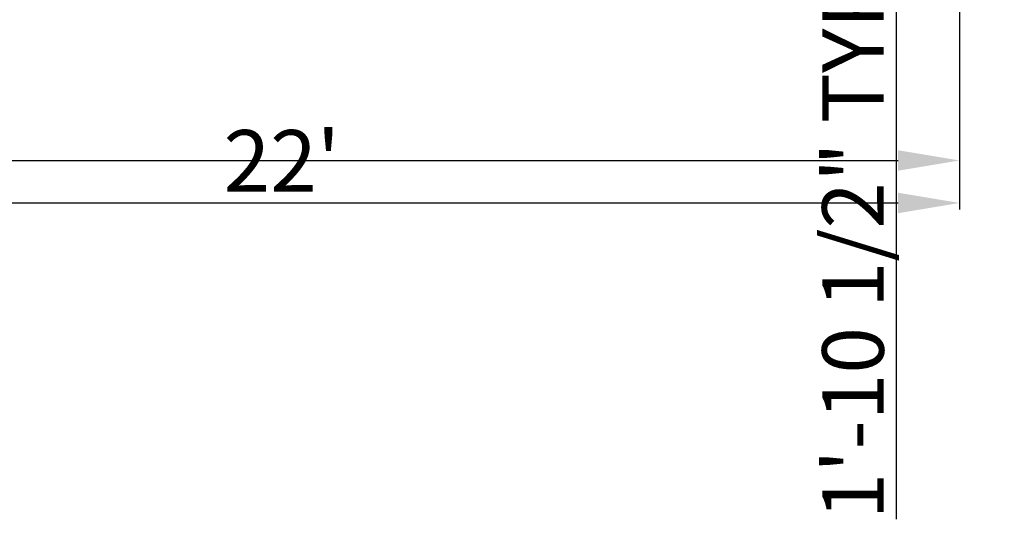
# Model space of a CAD drawing. Units: inches. Extents: x 2083 to 3317, y 1141 to 2115.
# Tile 117 of 256: x 2944 to 3136, y 1141 to 1238. Entities that reach past the tile are written whole.
import ezdxf

# ---------------------------------------------------------------- set-up
doc = ezdxf.new("R2010")
doc.units = ezdxf.units.IN
doc.layers.add('A-ANNO-DIMS', color=2, linetype='Continuous', lineweight=18)
doc.styles.get("Standard").update_dxf_attribs({"font": 'arial.ttf'})
doc.dimstyles.new('ISO-25', dxfattribs={"dimtxt": 12, "dimasz": 12, "dimexe": 1.25, "dimexo": 0.625, "dimtad": 1, "dimlunit": 3, "dimtxsty": 'Standard', "dimcen": 2.5, "dimadec": 0, "dimazin": 0, "dimtfac": 1, "dimtmove": 0, "dimatfit": 3, "dimfxl": 1, "dimarcsym": 0})

# ---------------------------------------------------------------- blocks, each defined once
blk = doc.blocks.new('*D10')
at = {"layer": 'A-ANNO-DIMS', "color": 0, "lineweight": -2, "transparency": 16777216}
for p, q in [((2862.96, 1262.64), (2862.96, 1201.38)), ((3126.96, 1262.64), (3126.96, 1201.38)), ((2874.96, 1202.63), (3114.96, 1202.63))]:
    blk.add_line(p, q, dxfattribs=at)
at = {"layer": 'A-ANNO-DIMS', "color": 0, "transparency": 16777216}
for points in [[(2874.96, 1204.63), (2874.96, 1200.63), (2862.96, 1202.63)], [(3114.96, 1204.63), (3114.96, 1200.63), (3126.96, 1202.63)]]:
    blk.add_solid(points, dxfattribs=at)
at = {"layer": 'Defpoints', "color": 0, "transparency": 16777216}
for p in [(2862.96, 1263.26), (3126.96, 1263.26), (3126.96, 1202.63)]:
    blk.add_point(p, dxfattribs=at)
at = {"layer": 'A-ANNO-DIMS', "color": 0, "transparency": 16777216, "insert": (2994.96, 1209.28), "char_height": 12, "attachment_point": 5}
blk.add_mtext("22'", dxfattribs=at)
blk = doc.blocks.new('*D27')
at = {"layer": 'A-ANNO-DIMS', "color": 0, "lineweight": -2, "transparency": 16777216}
for p, q in [((3114.58, 1309.79), (3114.58, 1321.79)), ((3111.87, 1297.79), (3115.83, 1297.79)), ((3114.58, 1297.79), (3114.58, 1275.54)), ((3111.87, 1275.54), (3115.83, 1275.54)), ((3114.58, 1263.54), (3114.58, 1140.99))]:
    blk.add_line(p, q, dxfattribs=at)
at = {"layer": 'A-ANNO-DIMS', "color": 0, "transparency": 16777216}
for points in [[(3112.58, 1309.79), (3116.58, 1309.79), (3114.58, 1297.79)], [(3112.58, 1263.54), (3116.58, 1263.54), (3114.58, 1275.54)]]:
    blk.add_solid(points, dxfattribs=at)
at = {"layer": 'Defpoints', "color": 0, "transparency": 16777216}
for p in [(3111.24, 1297.79), (3111.24, 1275.54), (3114.58, 1275.54)]:
    blk.add_point(p, dxfattribs=at)
at = {"layer": 'A-ANNO-DIMS', "color": 0, "transparency": 16777216, "insert": (3107.75, 1196.26), "char_height": 12, "attachment_point": 5, "rotation": 90}
blk.add_mtext('1\'-10 1/2" TYP.', dxfattribs=at)
blk = doc.blocks.new('*D34')
at = {"layer": 'A-ANNO-DIMS', "color": 0, "lineweight": -2, "transparency": 16777216}
for p, q in [((2226.96, 1262.64), (2226.96, 1209.66)), ((3126.96, 1262.64), (3126.96, 1209.66)), ((2238.96, 1210.91), (3114.96, 1210.91))]:
    blk.add_line(p, q, dxfattribs=at)
at = {"layer": 'A-ANNO-DIMS', "color": 0, "transparency": 16777216}
for points in [[(2238.96, 1212.91), (2238.96, 1208.91), (2226.96, 1210.91)], [(3114.96, 1212.91), (3114.96, 1208.91), (3126.96, 1210.91)]]:
    blk.add_solid(points, dxfattribs=at)
at = {"layer": 'Defpoints', "color": 0, "transparency": 16777216}
for p in [(2226.96, 1263.26), (3126.96, 1263.26), (3126.96, 1210.91)]:
    blk.add_point(p, dxfattribs=at)
at = {"layer": 'A-ANNO-DIMS', "color": 0, "transparency": 16777216, "insert": (2676.96, 1217.66), "char_height": 12, "attachment_point": 5}
blk.add_mtext('75\'-0"', dxfattribs=at)

msp = doc.modelspace()

# ---------------------------------------------------------------- dimensions: what is measured, and where the dimension line sits
at = {"layer": 'A-ANNO-DIMS'}
dim = msp.add_linear_dim(base=(3114.578, 1275.54), p1=(3111.24, 1297.794), p2=(3111.24, 1275.54), angle=270, text='<> TYP.', dimstyle='ISO-25', override={"dimdec": 1, "dimlfac": 1, "dimrnd": 0, "dimzin": 1, "dimdsep": 46, "dimlunit": 4, "dimfrac": 2}, dxfattribs=at)
dim.commit()
dim.dimension.update_dxf_attribs({"geometry": '*D27', "text_midpoint": (3107.749, 1196.264)})
for base, p1, override, picture, middle in [((3126.96, 1210.911), (2226.96, 1263.261), {"dimdec": 1, "dimlfac": 1, "dimrnd": 0, "dimzin": 1, "dimdsep": 46, "dimlunit": 4, "dimfrac": 2}, '*D34', (2676.96, 1217.663)), ((3126.96, 1202.634), (2862.96, 1263.261), {"dimclrd": 0, "dimclre": 0, "dimclrt": 0}, '*D10', (2994.96, 1209.284))]:
    dim = msp.add_linear_dim(base=base, p1=p1, p2=(3126.96, 1263.261), dimstyle='ISO-25', override=override, dxfattribs=at)
    dim.commit()
    dim.dimension.update_dxf_attribs({"geometry": picture, "text_midpoint": middle})

doc.saveas('drawing.dxf')
